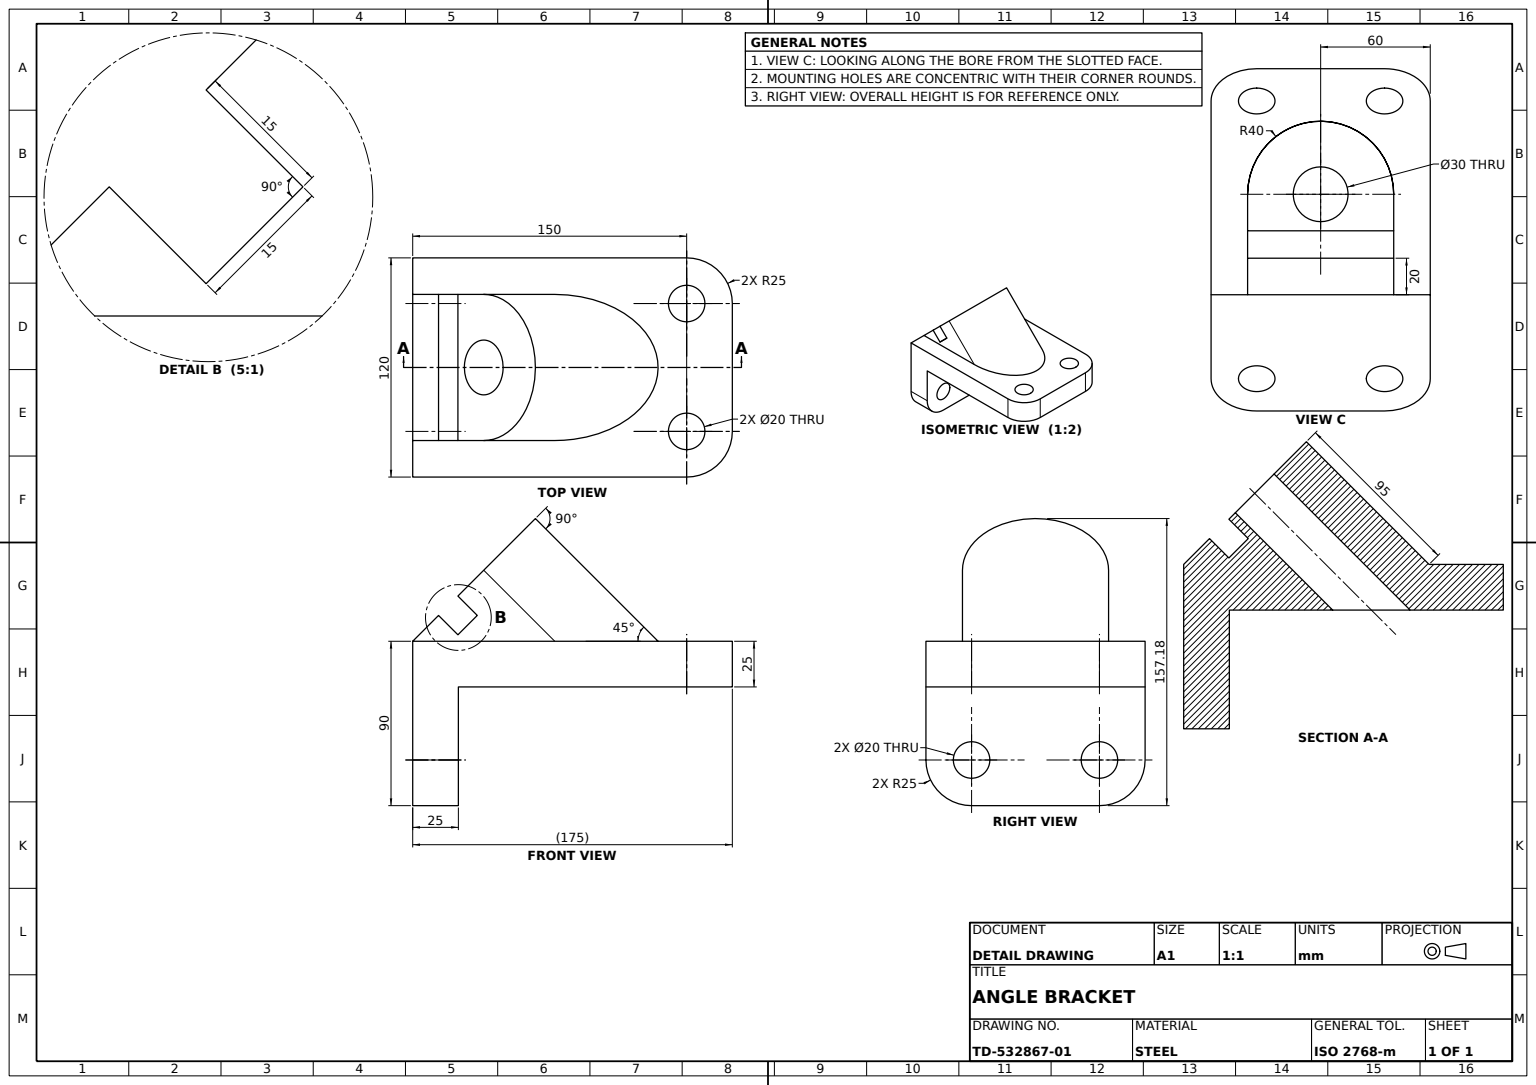
from build123d import *

# Parameters (mm, degrees)
UPRIGHT_PLATE_SKETCH_R          = 10
UPRIGHT_PLATE_DEPTH             = 25
BASE_PLATE_SKETCH_W             = 150
BASE_PLATE_SKETCH_H             = 25
BASE_PLATE_DEPTH                = 120
BASE_PLATE_CORNER_FILLETS_R25_R = 25
BASE_PLATE_HOLES_SKETCH_R       = 10
BASE_PLATE_HOLES_DEPTH          = 206.730406114
WEDGE_SUPPORT_DEPTH             = 60
LUG_PROFILE_CUT_REACH           = 227.051
LUG_PROFILE_SKETCH_R            = 15
LUG_BORE_SKETCH_R               = 15
LUG_BORE_DEPTH                  = 226.05084201
LUG_SLOT_SKETCH_W               = 80
LUG_SLOT_SKETCH_H               = 15
LUG_SLOT_15X20_DEPTH            = 15


with BuildPart() as part:
    # Upright Plate Sketch → Upright Plate (new body)
    with BuildSketch(Plane.XY):
        with BuildLine():
            Line((-60, 45), (60, 45))
            Line((60, 45), (60, -20))
            ThreePointArc((60, -20), (52.67766953, -37.67766953), (35, -45))
            Line((35, -45), (-35, -45))
            ThreePointArc((-35, -45), (-52.67766953, -37.67766953), (-60, -20))
            Line((-60, -20), (-60, 45))
        make_face()
        with Locations((-35, -20)):
            Circle(UPRIGHT_PLATE_SKETCH_R, mode=Mode.SUBTRACT)
        with Locations((35, -20)):
            Circle(UPRIGHT_PLATE_SKETCH_R, mode=Mode.SUBTRACT)
    extrude(amount=-UPRIGHT_PLATE_DEPTH)

    # Base Plate Sketch → Base Plate (add)
    with BuildSketch(Plane(origin=(60, 0, 0), x_dir=(0, 0, -1), z_dir=(1, 0, 0))):
        with Locations((100, 32.5)):
            Rectangle(BASE_PLATE_SKETCH_W, BASE_PLATE_SKETCH_H)
    extrude(amount=-BASE_PLATE_DEPTH)

    # Base Plate Corner Fillets R25
    base_plate_corner_fillets_r25_edges = [part.edges().sort_by_distance(p)[0] for p in [
        (-60, 32.5, -175),
        (60, 32.5, -175),
    ]]
    fillet(base_plate_corner_fillets_r25_edges, radius=BASE_PLATE_CORNER_FILLETS_R25_R)

    # Base Plate Holes Sketch → Base Plate Holes (cut, through all)
    with BuildSketch(Plane(origin=(0, 45, 0), x_dir=(1, 0, 0), z_dir=(0, 1, 0))):
        with Locations(Location((35, 150, 0), (0, 0, 270))):
            Circle(BASE_PLATE_HOLES_SKETCH_R)
        with Locations(Location((-35, 150, 0), (0, 0, 270))):
            Circle(BASE_PLATE_HOLES_SKETCH_R)
    extrude(amount=-BASE_PLATE_HOLES_DEPTH, mode=Mode.SUBTRACT)

    # Wedge Support Sketch → Wedge Support (add, symmetric)
    with BuildSketch(Plane(origin=(0, 0, 0), x_dir=(0, 0, -1), z_dir=(1, 0, 0))):
        Polygon((134.350288425, 45), (67.175144213, 112.175144213), (0, 45), align=None)
    extrude(amount=WEDGE_SUPPORT_DEPTH, both=True)

    # Lug Profile Cut: up to this face of the body (flat: up to its plane)
    lug_profile_cut_end = Plane(part.part.faces().sort_by_distance((0, 45, -154.419772532))[0])
    # Lug Profile Sketch → Lug Profile Cut (cut, up to the picked face)
    with BuildSketch(Plane(origin=(0, 22.5, 22.5), x_dir=(1, 0, 0), z_dir=(0, 0.7071067811865485, 0.7071067811865467)), mode=Mode.PRIVATE) as lug_profile_cut_sk1:
        with BuildLine():
            Line((-40, 31.819805153), (-40, 86.819805153))
            ThreePointArc((-40, 86.819805153), (-28.284271247, 115.104076401), (0, 126.819805153))
            Line((0, 126.819805153), (-60, 126.819805153))
            Line((-60, 126.819805153), (-60, 31.819805153))
            Line((-60, 31.819805153), (-40, 31.819805153))
        make_face()
    lug_profile_cut_tool1 = split(extrude(lug_profile_cut_sk1.sketch, amount=-LUG_PROFILE_CUT_REACH, mode=Mode.PRIVATE), bisect_by=lug_profile_cut_end, keep=Keep.BOTH, mode=Mode.PRIVATE)
    # Lug Profile Sketch → Lug Profile Cut (cut, up to the picked face)
    with BuildSketch(Plane(origin=(0, 22.5, 22.5), x_dir=(1, 0, 0), z_dir=(0, 0.7071067811865485, 0.7071067811865467)), mode=Mode.PRIVATE) as lug_profile_cut_sk2:
        with BuildLine():
            Line((60, 126.819805153), (0, 126.819805153))
            ThreePointArc((0, 126.819805153), (28.284271247, 115.104076401), (40, 86.819805153))
            Line((40, 86.819805153), (40, 31.819805153))
            Line((40, 31.819805153), (60, 31.819805153))
            Line((60, 31.819805153), (60, 126.819805153))
        make_face()
    lug_profile_cut_tool2 = split(extrude(lug_profile_cut_sk2.sketch, amount=-LUG_PROFILE_CUT_REACH, mode=Mode.PRIVATE), bisect_by=lug_profile_cut_end, keep=Keep.BOTH, mode=Mode.PRIVATE)
    # Lug Profile Sketch → Lug Profile Cut (cut, up to the picked face)
    with BuildSketch(Plane(origin=(0, 22.5, 22.5), x_dir=(1, 0, 0), z_dir=(0, 0.7071067811865485, 0.7071067811865467)), mode=Mode.PRIVATE) as lug_profile_cut_sk3:
        with Locations(Location((0, 86.819805153, 0), (0, 0, 270))):
            Circle(LUG_PROFILE_SKETCH_R)
    lug_profile_cut_tool3 = split(extrude(lug_profile_cut_sk3.sketch, amount=-LUG_PROFILE_CUT_REACH, mode=Mode.PRIVATE), bisect_by=lug_profile_cut_end, keep=Keep.BOTH, mode=Mode.PRIVATE)
    add(lug_profile_cut_tool1.solids().sort_by(Axis((-47.101904, 82.761408, -37.761408), (0, -0.7071067811865485, -0.7071067811865467)))[0], mode=Mode.SUBTRACT)
    add(lug_profile_cut_tool2.solids().sort_by(Axis((47.101904, 82.761408, -37.761408), (0, -0.7071067811865485, -0.7071067811865467)))[0], mode=Mode.SUBTRACT)
    add(lug_profile_cut_tool3.solids().sort_by(Axis((0, 83.890873, -38.890873), (0, -0.7071067811865485, -0.7071067811865467)))[0], mode=Mode.SUBTRACT)

    # Lug Bore Sketch → Lug Bore (cut, through all)
    with BuildSketch(Plane(origin=(0, 22.5, 22.5), x_dir=(1, 0, 0), z_dir=(0, 0.7071067811865485, 0.7071067811865467))):
        with Locations(Location((0, 86.819805153, 0), (0, 0, 270))):
            Circle(LUG_BORE_SKETCH_R)
    extrude(amount=-LUG_BORE_DEPTH, mode=Mode.SUBTRACT)

    # Lug Slot Sketch → Lug Slot 15x20 (cut)
    with BuildSketch(Plane(origin=(0, 22.5, 22.5), x_dir=(1, 0, 0), z_dir=(0, 0.7071067811865485, 0.7071067811865467))):
        with Locations((0, 59.319805153)):
            Rectangle(LUG_SLOT_SKETCH_W, LUG_SLOT_SKETCH_H)
    extrude(amount=-LUG_SLOT_15X20_DEPTH, mode=Mode.SUBTRACT)


solid = part.part
